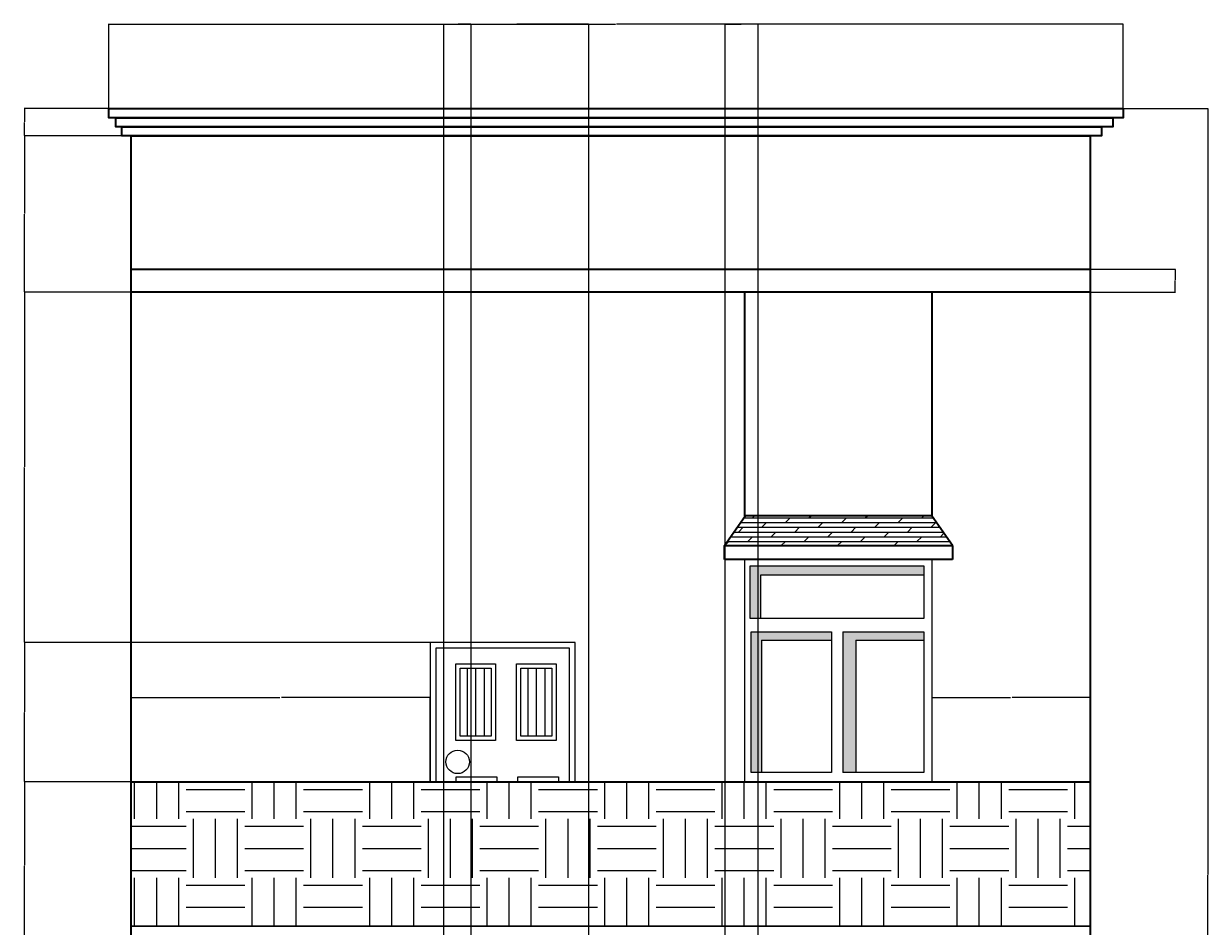
# Model space of a CAD drawing. Units: inches. Extents: x 1722 to 2362, y 1673 to 2617.
# Tile 2 of 2: x 1722 to 2362, y 2129 to 2617. Entities that reach past the tile are written whole.
import ezdxf

# ---------------------------------------------------------------- set-up
doc = ezdxf.new("R2010")
doc.units = ezdxf.units.IN
for name, color, linetype, lineweight in [('A-ANNO-DIMS', 2, 'Continuous', 18), ('A-DOOR', 3, 'Continuous', 25), ('A-FLOR', 7, 'Continuous', 30), ('A-GLAZ', 4, 'Continuous', 25), ('A-GLAZ-PATT', 8, 'Continuous', 13), ('A-ROOF', 7, 'Continuous', 35), ('A-ROOF-PATT', 8, 'Continuous', 13), ('A-WALL', 7, 'Continuous', 35), ('A-WALL-PATT', 8, 'Continuous', 13)]:
    doc.layers.add(name, color=color, linetype=linetype, lineweight=lineweight)
doc.styles.get("Standard").update_dxf_attribs({"font": 'arial.ttf'})
doc.dimstyles.get("Standard").update_dxf_attribs({"dimtxt": 0.18, "dimasz": 0.18, "dimexe": 0.18, "dimexo": 0.0625, "dimgap": 0.09, "dimtad": 0, "dimtih": 1, "dimtoh": 1, "dimdec": 4, "dimzin": 0, "dimdsep": 46, "dimtxsty": 'Standard', "dimcen": 0.09, "dimadec": 0, "dimazin": 0, "dimtfac": 1, "dimtdec": 4, "dimtofl": 0, "dimtmove": 0, "dimatfit": 3, "dimfxl": 1, "dimtolj": 1, "dimtzin": 0, "dimarcsym": 0})

# ---------------------------------------------------------------- blocks, each defined once
blk = doc.blocks.new('DOOR-PANEL-FLUTED')
for p, q in [((6.1, 39.03), (6.1, 2.33)), ((10.76, 39.03), (10.76, 2.33)), ((15.43, 39.03), (15.43, 2.33))]:
    blk.add_line(p, q)
for points in [[(0, 41.36), (21.52, 41.36), (21.52, 0), (0, 0)], [(2.33, 39.03), (19.19, 39.03), (19.19, 2.33), (2.33, 2.33)]]:
    blk.add_lwpolyline(points, close=True)
blk = doc.blocks.new('WIN-TWIN-TRANSOM')
for p, q in [((101.33, 120.15), (0, 120.15)), ((0, 120.15), (0, 0)), ((101.33, 0), (101.33, 120.15)), ((8.83, 88.28), (8.83, 111.99)), ((8.83, 111.99), (96.81, 111.99)), ((47.03, 81.23), (47.03, 5.04)), ((53.04, 81.23), (53.04, 5.04)), ((9.1, 76.71), (9.1, 5.04)), ((9.1, 76.71), (47.03, 76.71)), ((60.23, 76.71), (60.23, 5.04)), ((60.23, 76.71), (96.88, 76.71))]:
    blk.add_line(p, q)
blk.add_lwpolyline([(3.1, 116.89), (96.81, 116.89), (96.81, 88.28), (3.1, 88.28)], close=True)
for points in [[(47.03, 5.04), (3.67, 5.04), (3.67, 81.23), (47.03, 81.23)], [(53.04, 81.23), (96.88, 81.23), (96.88, 5.04), (53.04, 5.04)]]:
    blk.add_lwpolyline(points)
blk = doc.blocks.new('WIN-HOOD')
for p, q in [((0, 7.63), (11.4, 23.91)), ((11.4, 23.91), (111.91, 23.91)), ((123.31, 7.63), (111.91, 23.91)), ((0, 7.63), (123.31, 7.63)), ((0, 0), (0, 7.63)), ((123.31, 7.63), (123.31, 0)), ((123.31, 0), (0, 0))]:
    blk.add_line(p, q)
blk = doc.blocks.new('*D10')
at = {"layer": 'A-ANNO-DIMS', "color": 0, "lineweight": -2, "transparency": 16777216}
for p, q in [((1768.12, 2570.79), (1768.12, 2616.61)), ((1768.3, 2616.43), (2041.83, 2616.43)), ((2315.94, 2616.43), (2042.41, 2616.43)), ((2316.12, 2570.79), (2316.12, 2616.61))]:
    blk.add_line(p, q, dxfattribs=at)
at = {"layer": 'A-ANNO-DIMS', "color": 0, "transparency": 16777216}
for points in [[(1768.3, 2616.46), (1768.3, 2616.4), (1768.12, 2616.43)], [(2315.94, 2616.46), (2315.94, 2616.4), (2316.12, 2616.43)]]:
    blk.add_solid(points, dxfattribs=at)
at = {"layer": 'Defpoints', "color": 0, "transparency": 16777216}
for p in [(2316.12, 2616.43), (1768.12, 2570.73), (2316.12, 2570.73)]:
    blk.add_point(p, dxfattribs=at)
at = {"layer": 'A-ANNO-DIMS', "color": 0, "transparency": 16777216, "insert": (2042.12, 2616.43), "char_height": 0.18, "attachment_point": 5}
blk.add_mtext('\\A1;548', dxfattribs=at)
blk = doc.blocks.new('*D11')
at = {"layer": 'A-ANNO-DIMS', "color": 0, "lineweight": -2, "transparency": 16777216}
for p, q in [((2316.19, 2570.73), (2362, 2570.73)), ((2361.82, 2570.55), (2361.82, 2156.86)), ((2361.82, 1742.81), (2361.82, 2156.5)), ((2298.54, 1742.63), (2362, 1742.63))]:
    blk.add_line(p, q, dxfattribs=at)
at = {"layer": 'A-ANNO-DIMS', "color": 0, "transparency": 16777216}
for points in [[(2361.79, 2570.55), (2361.85, 2570.55), (2361.82, 2570.73)], [(2361.79, 1742.81), (2361.85, 1742.81), (2361.82, 1742.63)]]:
    blk.add_solid(points, dxfattribs=at)
at = {"layer": 'Defpoints', "color": 0, "transparency": 16777216}
for p in [(2316.12, 2570.73), (2361.82, 2570.73), (2298.48, 1742.63)]:
    blk.add_point(p, dxfattribs=at)
at = {"layer": 'A-ANNO-DIMS', "color": 0, "transparency": 16777216, "insert": (2361.82, 2156.68), "char_height": 0.18, "attachment_point": 5}
blk.add_mtext('\\A1;828.1', dxfattribs=at)
blk = doc.blocks.new('*D14')
at = {"layer": 'A-ANNO-DIMS', "color": 0, "lineweight": -2, "transparency": 16777216}
for p, q in [((1779.99, 2206.79), (1722.24, 2206.79)), ((1722.42, 2206.61), (1722.42, 2161.79)), ((1722.42, 2116.6), (1722.42, 2161.42)), ((1779.99, 2116.42), (1722.24, 2116.42))]:
    blk.add_line(p, q, dxfattribs=at)
at = {"layer": 'A-ANNO-DIMS', "color": 0, "transparency": 16777216}
for points in [[(1722.39, 2206.61), (1722.45, 2206.61), (1722.42, 2206.79)], [(1722.39, 2116.6), (1722.45, 2116.6), (1722.42, 2116.42)]]:
    blk.add_solid(points, dxfattribs=at)
at = {"layer": 'Defpoints', "color": 0, "transparency": 16777216}
for p in [(1722.42, 2206.79), (1780.05, 2206.79), (1780.05, 2116.42)]:
    blk.add_point(p, dxfattribs=at)
at = {"layer": 'A-ANNO-DIMS', "color": 0, "transparency": 16777216, "insert": (1722.42, 2161.6), "char_height": 0.18, "attachment_point": 5}
blk.add_mtext('\\A1;90.38', dxfattribs=at)
blk = doc.blocks.new('*D16')
at = {"layer": 'A-ANNO-DIMS', "color": 0, "lineweight": -2, "transparency": 16777216}
for p, q in [((1941.67, 2282.13), (1722.24, 2282.13)), ((1722.42, 2281.95), (1722.42, 2244.64)), ((1722.42, 2206.97), (1722.42, 2244.28)), ((1941.67, 2206.79), (1722.24, 2206.79))]:
    blk.add_line(p, q, dxfattribs=at)
at = {"layer": 'A-ANNO-DIMS', "color": 0, "transparency": 16777216}
for points in [[(1722.39, 2281.95), (1722.45, 2281.95), (1722.42, 2282.13)], [(1722.39, 2206.97), (1722.45, 2206.97), (1722.42, 2206.79)]]:
    blk.add_solid(points, dxfattribs=at)
at = {"layer": 'Defpoints', "color": 0, "transparency": 16777216}
for p in [(1722.42, 2282.13), (1941.73, 2282.13), (1941.73, 2206.79)]:
    blk.add_point(p, dxfattribs=at)
at = {"layer": 'A-ANNO-DIMS', "color": 0, "transparency": 16777216, "insert": (1722.42, 2244.46), "char_height": 0.18, "attachment_point": 5}
blk.add_mtext('\\A1;75.34', dxfattribs=at)
blk = doc.blocks.new('*D17')
at = {"layer": 'A-ANNO-DIMS', "color": 0, "lineweight": -2, "transparency": 16777216}
for p, q in [((1779.99, 2471.6), (1722.24, 2471.6)), ((1722.42, 2471.42), (1722.42, 2377.05)), ((1722.42, 2282.31), (1722.42, 2376.69)), ((1941.67, 2282.13), (1722.24, 2282.13))]:
    blk.add_line(p, q, dxfattribs=at)
at = {"layer": 'A-ANNO-DIMS', "color": 0, "transparency": 16777216}
for points in [[(1722.39, 2471.42), (1722.45, 2471.42), (1722.42, 2471.6)], [(1722.39, 2282.31), (1722.45, 2282.31), (1722.42, 2282.13)]]:
    blk.add_solid(points, dxfattribs=at)
at = {"layer": 'Defpoints', "color": 0, "transparency": 16777216}
for p in [(1722.42, 2471.6), (1780.05, 2471.6), (1941.73, 2282.13)]:
    blk.add_point(p, dxfattribs=at)
at = {"layer": 'A-ANNO-DIMS', "color": 0, "transparency": 16777216, "insert": (1722.42, 2376.87), "char_height": 0.18, "attachment_point": 5}
blk.add_mtext('\\A1;189.47', dxfattribs=at)
blk = doc.blocks.new('*D18')
at = {"layer": 'A-ANNO-DIMS', "color": 0, "lineweight": -2, "transparency": 16777216}
for p, q in [((1779.99, 2555.98), (1722.24, 2555.98)), ((1722.42, 2555.8), (1722.42, 2513.97)), ((1722.42, 2471.78), (1722.42, 2513.61)), ((1779.99, 2471.6), (1722.24, 2471.6))]:
    blk.add_line(p, q, dxfattribs=at)
at = {"layer": 'A-ANNO-DIMS', "color": 0, "transparency": 16777216}
for points in [[(1722.39, 2555.8), (1722.45, 2555.8), (1722.42, 2555.98)], [(1722.39, 2471.78), (1722.45, 2471.78), (1722.42, 2471.6)]]:
    blk.add_solid(points, dxfattribs=at)
at = {"layer": 'Defpoints', "color": 0, "transparency": 16777216}
for p in [(1722.42, 2555.98), (1780.05, 2555.98), (1780.05, 2471.6)]:
    blk.add_point(p, dxfattribs=at)
at = {"layer": 'A-ANNO-DIMS', "color": 0, "transparency": 16777216, "insert": (1722.42, 2513.79), "char_height": 0.18, "attachment_point": 5}
blk.add_mtext('\\A1;84.38', dxfattribs=at)
blk = doc.blocks.new('*D19')
at = {"layer": 'A-ANNO-DIMS', "color": 0, "lineweight": -2, "transparency": 16777216}
for p, q in [((2298.54, 2483.98), (2344.36, 2483.98)), ((2344.18, 2483.8), (2344.18, 2477.97)), ((2344.18, 2471.78), (2344.18, 2477.61)), ((2298.54, 2471.6), (2344.36, 2471.6))]:
    blk.add_line(p, q, dxfattribs=at)
at = {"layer": 'A-ANNO-DIMS', "color": 0, "transparency": 16777216}
for points in [[(2344.15, 2483.8), (2344.21, 2483.8), (2344.18, 2483.98)], [(2344.15, 2471.78), (2344.21, 2471.78), (2344.18, 2471.6)]]:
    blk.add_solid(points, dxfattribs=at)
at = {"layer": 'Defpoints', "color": 0, "transparency": 16777216}
for p in [(2298.48, 2483.98), (2298.48, 2471.6), (2344.18, 2471.6)]:
    blk.add_point(p, dxfattribs=at)
at = {"layer": 'A-ANNO-DIMS', "color": 0, "transparency": 16777216, "insert": (2344.18, 2477.79), "char_height": 0.18, "attachment_point": 5}
blk.add_mtext('\\A1;12.378', dxfattribs=at)
blk = doc.blocks.new('*D20')
at = {"layer": 'A-ANNO-DIMS', "color": 0, "lineweight": -2, "transparency": 16777216}
for p, q in [((1768.05, 2570.73), (1722.24, 2570.73)), ((1722.42, 2570.55), (1722.42, 2563.54)), ((1722.42, 2556.16), (1722.42, 2563.17)), ((1779.99, 2555.98), (1722.24, 2555.98))]:
    blk.add_line(p, q, dxfattribs=at)
at = {"layer": 'A-ANNO-DIMS', "color": 0, "transparency": 16777216}
for points in [[(1722.39, 2570.55), (1722.45, 2570.55), (1722.42, 2570.73)], [(1722.39, 2556.16), (1722.45, 2556.16), (1722.42, 2555.98)]]:
    blk.add_solid(points, dxfattribs=at)
at = {"layer": 'Defpoints', "color": 0, "transparency": 16777216}
for p in [(1722.42, 2570.73), (1768.12, 2570.73), (1780.05, 2555.98)]:
    blk.add_point(p, dxfattribs=at)
at = {"layer": 'A-ANNO-DIMS', "color": 0, "transparency": 16777216, "insert": (1722.42, 2563.36), "char_height": 0.18, "attachment_point": 5}
blk.add_mtext('\\A1;14.75', dxfattribs=at)
blk = doc.blocks.new('*D21')
at = {"layer": 'A-ANNO-DIMS', "color": 0, "lineweight": -2, "transparency": 16777216}
for p, q in [((1780.05, 2206.86), (1780.05, 2252.67)), ((1780.23, 2252.49), (1860.44, 2252.49)), ((1941.55, 2252.49), (1861.35, 2252.49)), ((1941.73, 2206.86), (1941.73, 2252.67))]:
    blk.add_line(p, q, dxfattribs=at)
at = {"layer": 'A-ANNO-DIMS', "color": 0, "transparency": 16777216}
for points in [[(1780.23, 2252.52), (1780.23, 2252.46), (1780.05, 2252.49)], [(1941.55, 2252.52), (1941.55, 2252.46), (1941.73, 2252.49)]]:
    blk.add_solid(points, dxfattribs=at)
at = {"layer": 'Defpoints', "color": 0, "transparency": 16777216}
for p in [(1941.73, 2252.49), (1780.05, 2206.79), (1941.73, 2206.79)]:
    blk.add_point(p, dxfattribs=at)
at = {"layer": 'A-ANNO-DIMS', "color": 0, "transparency": 16777216, "insert": (1860.89, 2252.49), "char_height": 0.18, "attachment_point": 5}
blk.add_mtext('\\A1;161.68', dxfattribs=at)
blk = doc.blocks.new('*D22')
at = {"layer": 'A-ANNO-DIMS', "color": 0, "lineweight": -2, "transparency": 16777216}
for p, q in [((2212.85, 2206.86), (2212.85, 2252.67)), ((2213.03, 2252.49), (2255.27, 2252.49)), ((2298.3, 2252.49), (2256.06, 2252.49)), ((2298.48, 2206.86), (2298.48, 2252.67))]:
    blk.add_line(p, q, dxfattribs=at)
at = {"layer": 'A-ANNO-DIMS', "color": 0, "transparency": 16777216}
for points in [[(2213.03, 2252.52), (2213.03, 2252.46), (2212.85, 2252.49)], [(2298.3, 2252.52), (2298.3, 2252.46), (2298.48, 2252.49)]]:
    blk.add_solid(points, dxfattribs=at)
at = {"layer": 'Defpoints', "color": 0, "transparency": 16777216}
for p in [(2298.48, 2252.49), (2212.85, 2206.79), (2298.48, 2206.79)]:
    blk.add_point(p, dxfattribs=at)
at = {"layer": 'A-ANNO-DIMS', "color": 0, "transparency": 16777216, "insert": (2255.66, 2252.49), "char_height": 0.18, "attachment_point": 5}
blk.add_mtext('\\A1;85.63', dxfattribs=at)
blk = doc.blocks.new('*D26')
at = {"layer": 'A-ANNO-DIMS', "color": 0, "lineweight": -2, "transparency": 16777216}
for p, q in [((1949.04, 1927.01), (1949.04, 2616.61)), ((1949.22, 2616.43), (1987.86, 2616.43)), ((2027.15, 2616.43), (1988.51, 2616.43)), ((2027.33, 1927.01), (2027.33, 2616.61))]:
    blk.add_line(p, q, dxfattribs=at)
at = {"layer": 'A-ANNO-DIMS', "color": 0, "transparency": 16777216}
for points in [[(1949.22, 2616.46), (1949.22, 2616.4), (1949.04, 2616.43)], [(2027.15, 2616.46), (2027.15, 2616.4), (2027.33, 2616.43)]]:
    blk.add_solid(points, dxfattribs=at)
at = {"layer": 'Defpoints', "color": 0, "transparency": 16777216}
for p in [(2027.33, 2616.43), (1949.04, 1926.94), (2027.33, 1926.94)]:
    blk.add_point(p, dxfattribs=at)
at = {"layer": 'A-ANNO-DIMS', "color": 0, "transparency": 16777216, "insert": (1988.18, 2616.43), "char_height": 0.18, "attachment_point": 5}
blk.add_mtext('\\A1;78.3', dxfattribs=at)
blk = doc.blocks.new('*D32')
at = {"layer": 'A-ANNO-DIMS', "color": 0, "lineweight": -2, "transparency": 16777216}
for p, q in [((1949.04, 1802.69), (1949.04, 2616.61)), ((1949.22, 2616.43), (1955.98, 2616.43)), ((1963.65, 2616.43), (1956.89, 2616.43)), ((1963.83, 1862.54), (1963.83, 2616.61))]:
    blk.add_line(p, q, dxfattribs=at)
at = {"layer": 'A-ANNO-DIMS', "color": 0, "transparency": 16777216}
for points in [[(1949.22, 2616.46), (1949.22, 2616.4), (1949.04, 2616.43)], [(1963.65, 2616.46), (1963.65, 2616.4), (1963.83, 2616.43)]]:
    blk.add_solid(points, dxfattribs=at)
at = {"layer": 'Defpoints', "color": 0, "transparency": 16777216}
for p in [(1963.83, 2616.43), (1963.83, 1862.48), (1949.04, 1802.63)]:
    blk.add_point(p, dxfattribs=at)
at = {"layer": 'A-ANNO-DIMS', "color": 0, "transparency": 16777216, "insert": (1956.43, 2616.43), "char_height": 0.18, "attachment_point": 5}
blk.add_mtext('\\A1;14.794', dxfattribs=at)
blk = doc.blocks.new('*D36')
at = {"layer": 'A-ANNO-DIMS', "color": 0, "lineweight": -2, "transparency": 16777216}
for p, q in [((2101.13, 1857.91), (2101.13, 2616.61)), ((2101.31, 2616.43), (2109.67, 2616.43)), ((2118.65, 2616.43), (2110.3, 2616.43)), ((2118.83, 1857.91), (2118.83, 2616.61))]:
    blk.add_line(p, q, dxfattribs=at)
at = {"layer": 'A-ANNO-DIMS', "color": 0, "transparency": 16777216}
for points in [[(2101.31, 2616.46), (2101.31, 2616.4), (2101.13, 2616.43)], [(2118.65, 2616.46), (2118.65, 2616.4), (2118.83, 2616.43)]]:
    blk.add_solid(points, dxfattribs=at)
at = {"layer": 'Defpoints', "color": 0, "transparency": 16777216}
for p in [(2118.83, 2616.43), (2101.13, 1857.84), (2118.83, 1857.84)]:
    blk.add_point(p, dxfattribs=at)
at = {"layer": 'A-ANNO-DIMS', "color": 0, "transparency": 16777216, "insert": (2109.98, 2616.43), "char_height": 0.18, "attachment_point": 5}
blk.add_mtext('\\A1;17.7', dxfattribs=at)

msp = doc.modelspace()

# ---------------------------------------------------------------- hatches: boundary and pattern name
at = {"layer": 'A-GLAZ-PATT'}
h = msp.add_hatch(color=256, dxfattribs=at)
h.dxf.hatch_style = 1
h.paths.add_polyline_path([(2127.935, 1934.5566), (2165.8618, 1934.5566), (2165.8618, 1939.0711), (2122.497, 1939.0711), (2122.497, 1862.8793), (2127.935, 1862.8793)])
h.paths.add_polyline_path([(2215.6423, 1974.7364), (2121.926, 1974.7364), (2121.926, 1946.1274), (2127.6599, 1946.1274), (2127.6599, 1969.8374), (2215.6423, 1969.8374)])
h.paths.add_polyline_path([(2179.0618, 1934.5566), (2215.7078, 1934.5566), (2215.7078, 1939.0711), (2171.8684, 1939.0711), (2171.8684, 1862.8793), (2179.0618, 1862.8793)])
h.paths.add_polyline_path([(2120.6292, 2283.5064), (2158.556, 2283.5064), (2158.556, 2288.0209), (2115.1912, 2288.0209), (2115.1912, 2211.8291), (2120.6292, 2211.8291)])
h.paths.add_polyline_path([(2171.756, 2283.5064), (2208.402, 2283.5064), (2208.402, 2288.0209), (2164.5626, 2288.0209), (2164.5626, 2211.8291), (2171.756, 2211.8291)])
h.paths.add_polyline_path([(2120.3541, 2318.7873), (2208.3365, 2318.7873), (2208.3365, 2323.6862), (2114.6202, 2323.6862), (2114.6202, 2295.0772), (2120.3541, 2295.0772)])
h = msp.add_hatch(color=256, dxfattribs=at)
h.dxf.hatch_style = 1
h.set_gradient(color1=(99, 100, 102), color2=(0, 0, 0), name='INVCYLINDER')
h.paths.add_polyline_path([(2127.935, 1934.5566), (2165.8618, 1934.5566), (2165.8618, 1939.0711), (2122.497, 1939.0711), (2122.497, 1862.8793), (2127.935, 1862.8793)])
h.paths.add_polyline_path([(2179.0618, 1934.5566), (2215.7078, 1934.5566), (2215.7078, 1939.0711), (2171.8684, 1939.0711), (2171.8684, 1862.8793), (2179.0618, 1862.8793)])
h.paths.add_polyline_path([(2127.6599, 1969.8374), (2215.6423, 1969.8374), (2215.6423, 1974.7364), (2121.926, 1974.7364), (2121.926, 1946.1274), (2127.6599, 1946.1274)])
h.paths.add_polyline_path([(2120.6292, 2283.5064), (2158.556, 2283.5064), (2158.556, 2288.0209), (2115.1912, 2288.0209), (2115.1912, 2211.8291), (2120.6292, 2211.8291)])
h.paths.add_polyline_path([(2171.756, 2283.5064), (2208.402, 2283.5064), (2208.402, 2288.0209), (2164.5626, 2288.0209), (2164.5626, 2211.8291), (2171.756, 2211.8291)])
h.paths.add_polyline_path([(2120.3541, 2318.7873), (2208.3365, 2318.7873), (2208.3365, 2323.6862), (2114.6202, 2323.6862), (2114.6202, 2295.0772), (2120.3541, 2295.0772)])
at = {"layer": 'A-ROOF-PATT'}
h = msp.add_hatch(dxfattribs=at)
h.set_pattern_fill('DOLMIT', color=256, scale=0.4)
h.paths.add_polyline_path([(2219.8784, 2001.9022), (2119.372, 2001.9022), (2107.9725, 1985.6219), (2231.2779, 1985.6219)])
h.paths.add_polyline_path([(2212.5726, 2350.8521), (2112.0662, 2350.8521), (2100.6667, 2334.5718), (2223.9721, 2334.5718)])
at = {"layer": 'A-WALL-PATT'}
h = msp.add_hatch(dxfattribs=at)
h.set_pattern_fill('EARTH', color=256, scale=5)
h.paths.add_polyline_path([(2298.4756, 2206.7935), (1780.0546, 2206.7935), (1780.0546, 2128.7935), (2298.4756, 2128.7935)])
h = msp.add_hatch(dxfattribs=at)
h.set_pattern_fill('EARTH', color=256, scale=5)
h.paths.add_polyline_path([(2298.4756, 2128.7935), (2298.4756, 2200.7935), (1849.8061, 2200.7935), (1849.8061, 2128.7935)])

# ---------------------------------------------------------------- linework, layer by layer
at = {"layer": 'A-DOOR'}
for p, q in [((2020.0261, 2282.1318), (1941.7304, 2282.1318)), ((1941.7304, 2282.1318), (1941.7304, 2206.7935)), ((2020.0261, 2206.7935), (2020.0261, 2282.1318)), ((1955.6635, 2206.7935), (1955.6635, 2209.5132)), ((1955.6635, 2209.5132), (1977.6163, 2209.5132)), ((1977.6163, 2209.5132), (1977.6163, 2206.7935)), ((1989.0119, 2206.7935), (1989.0119, 2209.5132)), ((1989.0119, 2209.5132), (2010.9647, 2209.5132)), ((2010.9647, 2209.5132), (2010.9647, 2206.7935))]:
    msp.add_line(p, q, dxfattribs=at)
msp.add_lwpolyline([(2017.0261, 2206.7935), (2017.0261, 2279.1318), (1944.7304, 2279.1318), (1944.7304, 2206.7935)], dxfattribs=at)
msp.add_circle((1956.524, 2217.6689), 6.3375, dxfattribs=at)
at = {"layer": 'A-FLOR'}
msp.add_line((1780.0546, 2128.7935), (2298.4756, 2128.7935), dxfattribs=at)
at = {"layer": 'A-ROOF'}
for p, q in [((1780.0546, 2555.9811), (2298.4756, 2555.9811)), ((1780.0546, 2483.9811), (2298.4756, 2483.9811)), ((1780.0546, 2471.6027), (2298.4756, 2471.6027))]:
    msp.add_line(p, q, dxfattribs=at)
for points in [[(1768.1171, 2570.7297), (2316.1231, 2570.7297), (2316.1231, 2565.803), (1768.1171, 2565.803)], [(1771.7546, 2565.803), (2310.5524, 2565.803), (2310.5524, 2560.8762), (1771.7546, 2560.8762)], [(1775.0735, 2560.8762), (2304.3942, 2560.8762), (2304.3942, 2555.9495), (1775.0735, 2555.9495)]]:
    msp.add_lwpolyline(points, close=True, dxfattribs=at)
at = {"layer": 'A-WALL'}
for p, q in [((1780.0546, 1742.6293), (1780.0546, 2555.9811)), ((2298.4756, 1742.6293), (2298.4756, 2555.9811)), ((2111.5244, 2471.6027), (2111.5244, 2350.0782)), ((2212.8505, 2350.4552), (2212.8505, 2471.6027)), ((1780.0546, 2206.7935), (2298.4756, 2206.7935))]:
    msp.add_line(p, q, dxfattribs=at)

# ---------------------------------------------------------------- block references
at = {"layer": 'A-DOOR'}
for p in [(1955.4922, 2229.2226), (1988.2772, 2229.2226)]:
    msp.add_blockref('DOOR-PANEL-FLUTED', p, dxfattribs=at)
at = {"layer": 'A-GLAZ'}
msp.add_blockref('WIN-TWIN-TRANSOM', (2111.5242, 2206.7938), dxfattribs=at)
at = {"layer": 'A-ROOF'}
msp.add_blockref('WIN-HOOD', (2100.6662, 2326.9448), dxfattribs=at)

# ---------------------------------------------------------------- dimensions: what is measured, and where the dimension line sits
at = {"layer": 'A-ANNO-DIMS'}
for base, p1, p2, override, picture, middle in [((2316.1231, 2616.4297), (1768.1171, 2570.7297), (2316.1231, 2570.7297), {"dimdec": 0, "dimlfac": 1, "dimrnd": 0, "dimzin": 0, "dimdsep": 46, "dimlunit": 2}, '*D10', (2042.1201, 2616.4297)), ((2027.3319, 2616.4297), (1949.0362, 1926.9442), (2027.3319, 1926.9442), {"dimdec": 1, "dimlfac": 1, "dimrnd": 0, "dimzin": 0, "dimdsep": 46, "dimlunit": 2}, '*D26', (1988.1841, 2616.4297)), ((1963.8298, 2616.4297), (1949.0362, 1802.6293), (1963.8298, 1862.4813), {"dimdec": 3, "dimlfac": 1, "dimrnd": 0, "dimzin": 0, "dimdsep": 46, "dimlunit": 2}, '*D32', (1956.433, 2616.4297)), ((2118.8302, 2616.4297), (2101.1312, 1857.8437), (2118.8302, 1857.8437), {"dimdec": 1, "dimlfac": 1, "dimrnd": 0, "dimzin": 0, "dimdsep": 46, "dimlunit": 2}, '*D36', (2109.9807, 2616.4297)), ((1941.7304, 2252.4935), (1780.0546, 2206.7935), (1941.7304, 2206.7935), {"dimdec": 2, "dimlfac": 1, "dimrnd": 0, "dimzin": 0, "dimdsep": 46, "dimlunit": 2}, '*D21', (1860.8925, 2252.4935))]:
    dim = msp.add_linear_dim(base=base, p1=p1, p2=p2, dimstyle='Standard', override=override, dxfattribs=at)
    dim.commit()
    dim.dimension.update_dxf_attribs({"geometry": picture, "text_midpoint": middle})
for base, p1, p2, angle, override, picture, middle in [((1722.4171, 2570.7297), (1780.0546, 2555.9811), (1768.1171, 2570.7297), 90, {"dimdec": 2, "dimlfac": 1, "dimrnd": 0, "dimzin": 0, "dimdsep": 46, "dimlunit": 2}, '*D20', (1722.4171, 2563.3554)), ((2361.8231, 2570.7297), (2298.4756, 1742.6293), (2316.1231, 2570.7297), 90, {"dimdec": 1, "dimlfac": 1, "dimrnd": 0, "dimzin": 0, "dimdsep": 46, "dimlunit": 2}, '*D11', (2361.8231, 2156.6795)), ((1722.4171, 2555.9811), (1780.0546, 2471.6027), (1780.0546, 2555.9811), 90, {"dimdec": 2, "dimlfac": 1, "dimrnd": 0, "dimzin": 0, "dimdsep": 46, "dimlunit": 2}, '*D18', (1722.4171, 2513.7919)), ((2344.1756, 2471.6027), (2298.4756, 2483.9811), (2298.4756, 2471.6027), 270, {"dimdec": 3, "dimlfac": 1, "dimrnd": 0, "dimzin": 0, "dimdsep": 46, "dimlunit": 2}, '*D19', (2344.1756, 2477.7919)), ((1722.4171, 2471.6027), (1941.7304, 2282.1318), (1780.0546, 2471.6027), 90, {"dimdec": 2, "dimlfac": 1, "dimrnd": 0, "dimzin": 0, "dimdsep": 46, "dimlunit": 2}, '*D17', (1722.4171, 2376.8672)), ((1722.4171, 2282.1318), (1941.7304, 2206.7935), (1941.7304, 2282.1318), 90, {"dimdec": 2, "dimlfac": 1, "dimrnd": 0, "dimzin": 0, "dimdsep": 46, "dimlunit": 2}, '*D16', (1722.4171, 2244.4627)), ((2298.4756, 2252.4935), (2212.8505, 2206.7935), (2298.4756, 2206.7935), 0, {"dimdec": 2, "dimlfac": 1, "dimrnd": 0, "dimzin": 0, "dimdsep": 46, "dimlunit": 2}, '*D22', (2255.663, 2252.4935)), ((1722.4171, 2206.7935), (1780.0546, 2116.4151), (1780.0546, 2206.7935), 90, {"dimdec": 2, "dimlfac": 1, "dimrnd": 0, "dimzin": 0, "dimdsep": 46, "dimlunit": 2}, '*D14', (1722.4171, 2161.6043))]:
    dim = msp.add_linear_dim(base=base, p1=p1, p2=p2, angle=angle, dimstyle='Standard', override=override, dxfattribs=at)
    dim.commit()
    dim.dimension.update_dxf_attribs({"geometry": picture, "text_midpoint": middle})

doc.saveas('drawing.dxf')
